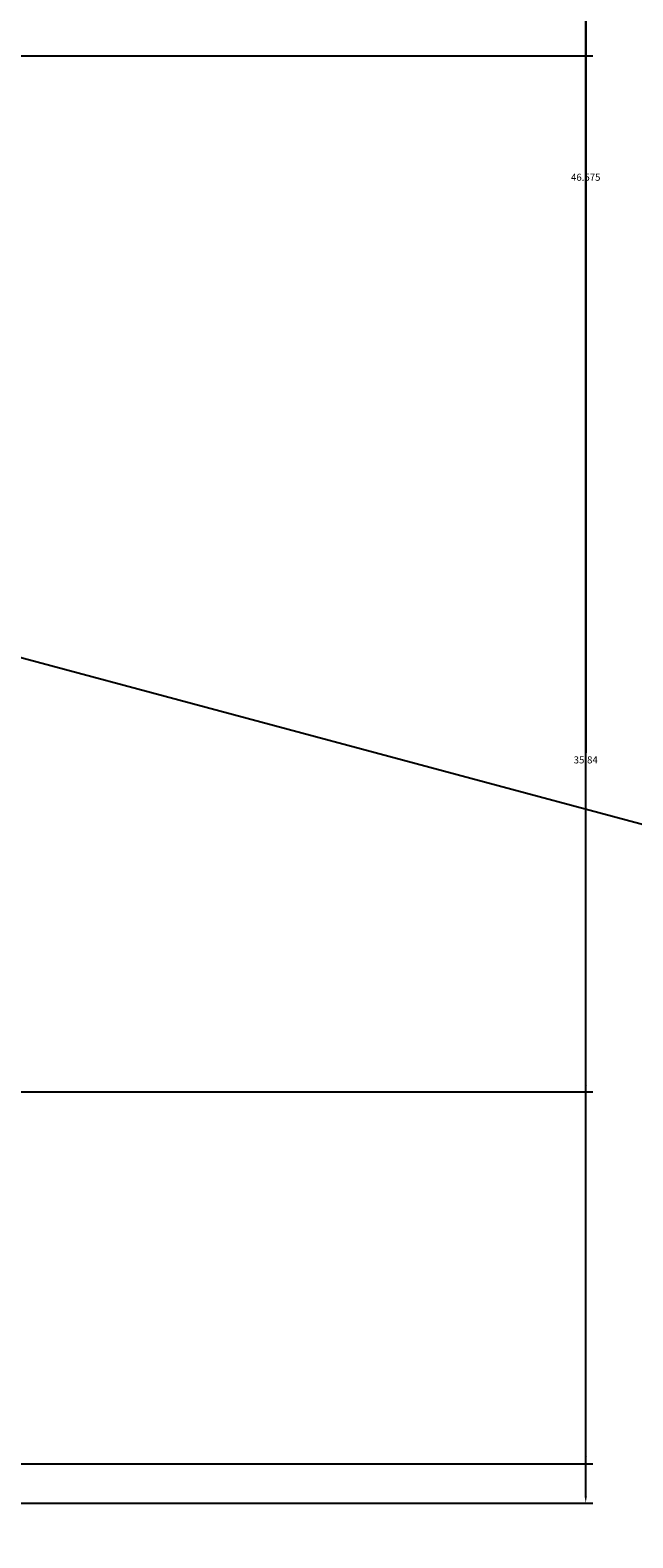
# Model space of a CAD drawing. Units: inches. Extents: x -12 to 334, y -10 to 186.
# Tile 72 of 77: x 282 to 297, y 45 to 83. Entities that reach past the tile are written whole.
import ezdxf
from ezdxf import colors
from ezdxf.entities.mleader import LeaderData, LeaderLine
from ezdxf.math import Vec2, Vec3

# ---------------------------------------------------------------- set-up
doc = ezdxf.new("R2010")
doc.units = ezdxf.units.IN
doc.header["$MEASUREMENT"] = 0
doc.layers.add('M-ANNO-TEXT', color=3, linetype='Continuous', lineweight=25)
doc.layers.add('M-DIMS', color=2, linetype='Continuous', lineweight=18)
doc.styles.get("Standard").update_dxf_attribs({"font": 'arial.ttf'})
doc.dimstyles.get("Standard").update_dxf_attribs({"dimtxt": 0.18, "dimasz": 0.18, "dimexe": 0.18, "dimexo": 0.0625, "dimgap": 0.09, "dimtad": 0, "dimtih": 1, "dimtoh": 1, "dimdec": 4, "dimzin": 0, "dimdsep": 46, "dimtxsty": 'Standard', "dimcen": 0.09, "dimadec": 0, "dimazin": 0, "dimtfac": 1, "dimtdec": 4, "dimtofl": 0, "dimtmove": 0, "dimatfit": 3, "dimfxl": 1, "dimtolj": 1, "dimtzin": 0, "dimarcsym": 0})

# ---------------------------------------------------------------- blocks, each defined once
blk = doc.blocks.new('*D17')
at = {"layer": 'Defpoints', "color": 0, "transparency": 16777216}
for p in [(106.177, 102.896), (105.892, 56.321), (295.976, 56.321)]:
    blk.add_point(p, dxfattribs=at)
at = {"layer": 'M-DIMS', "color": 0, "lineweight": -2, "transparency": 16777216}
for p, q in [((106.24, 102.896), (296.156, 102.896)), ((295.976, 102.716), (295.976, 79.79)), ((295.976, 56.501), (295.976, 79.426)), ((105.954, 56.321), (296.156, 56.321))]:
    blk.add_line(p, q, dxfattribs=at)
at = {"layer": 'M-DIMS', "color": 0, "transparency": 16777216}
for points in [[(295.946, 102.716), (296.006, 102.716), (295.976, 102.896)], [(295.946, 56.501), (296.006, 56.501), (295.976, 56.321)]]:
    blk.add_solid(points, dxfattribs=at)
at = {"layer": 'M-DIMS', "color": 0, "transparency": 16777216, "insert": (295.976, 79.608), "char_height": 0.18, "attachment_point": 5}
blk.add_mtext('\\A1;46.575', dxfattribs=at)
blk = doc.blocks.new('*D24')
at = {"layer": 'Defpoints', "color": 0, "transparency": 16777216}
for p in [(269.381, 137.943), (269.381, 45.854), (295.976, 45.854)]:
    blk.add_point(p, dxfattribs=at)
at = {"layer": 'M-DIMS', "color": 0, "lineweight": -2, "transparency": 16777216}
for p, q in [((269.443, 137.943), (296.156, 137.943)), ((295.976, 137.763), (295.976, 92.081)), ((295.976, 46.034), (295.976, 91.717)), ((269.443, 45.854), (296.156, 45.854))]:
    blk.add_line(p, q, dxfattribs=at)
at = {"layer": 'M-DIMS', "color": 0, "transparency": 16777216}
for points in [[(295.946, 137.763), (296.006, 137.763), (295.976, 137.943)], [(295.946, 46.034), (296.006, 46.034), (295.976, 45.854)]]:
    blk.add_solid(points, dxfattribs=at)
at = {"layer": 'M-DIMS', "color": 0, "transparency": 16777216, "insert": (295.976, 91.899), "char_height": 0.18, "attachment_point": 5}
blk.add_mtext('\\A1;92.09', dxfattribs=at)
blk = doc.blocks.new('*D38')
at = {"layer": 'Defpoints', "color": 0, "transparency": 16777216}
for p in [(247.935, 82.697), (247.935, 46.854), (295.976, 46.854)]:
    blk.add_point(p, dxfattribs=at)
at = {"layer": 'M-DIMS', "color": 0, "lineweight": -2, "transparency": 16777216}
for p, q in [((247.998, 82.697), (296.156, 82.697)), ((295.976, 82.517), (295.976, 64.957)), ((295.976, 47.034), (295.976, 64.594)), ((247.998, 46.854), (296.156, 46.854))]:
    blk.add_line(p, q, dxfattribs=at)
at = {"layer": 'M-DIMS', "color": 0, "transparency": 16777216}
for points in [[(295.946, 82.517), (296.006, 82.517), (295.976, 82.697)], [(295.946, 47.034), (296.006, 47.034), (295.976, 46.854)]]:
    blk.add_solid(points, dxfattribs=at)
at = {"layer": 'M-DIMS', "color": 0, "transparency": 16777216, "insert": (295.976, 64.775), "char_height": 0.18, "attachment_point": 5}
blk.add_mtext('\\A1;35.84', dxfattribs=at)
blk = doc.blocks.new('*D41')
at = {"layer": 'Defpoints', "color": 0, "transparency": 16777216}
for p in [(190.169, 91.899), (277.343, 68.515)]:
    blk.add_point(p, dxfattribs=at)
at = {"layer": 'M-DIMS', "color": 0, "lineweight": -2, "transparency": 16777216}
for p, q in [((190.079, 91.899), (190.259, 91.899)), ((190.169, 91.809), (190.169, 91.989)), ((329.648, 54.485), (277.517, 68.469)), ((329.828, 54.485), (329.648, 54.485))]:
    blk.add_line(p, q, dxfattribs=at)
at = {"layer": 'M-DIMS', "color": 0, "transparency": 16777216}
blk.add_solid([(277.525, 68.498), (277.509, 68.44), (277.343, 68.515)], dxfattribs=at)
at = {"layer": 'M-DIMS', "color": 0, "transparency": 16777216, "insert": (330.307, 54.485), "char_height": 0.18, "attachment_point": 5}
blk.add_mtext('\\A1;R90.26', dxfattribs=at)

msp = doc.modelspace()

# ---------------------------------------------------------------- dimensions: what is measured, and where the dimension line sits
at = {"layer": 'M-DIMS'}
for base, p1, p2, override, picture, middle in [((295.9756, 45.8541), (269.3808, 137.9435), (269.3808, 45.8541), {"dimdec": 2, "dimlfac": 1, "dimrnd": 0, "dimzin": 0, "dimdsep": 46, "dimlunit": 2}, '*D24', (295.9756, 91.8988)), ((295.9756, 56.3205), (106.1771, 102.8958), (105.8919, 56.3205), {"dimdec": 3, "dimlfac": 1, "dimrnd": 0, "dimzin": 0, "dimdsep": 46, "dimlunit": 2}, '*D17', (295.9756, 79.6082)), ((295.9756, 46.8541), (247.9354, 82.6969), (247.9354, 46.8541), {"dimdec": 2, "dimlfac": 1, "dimrnd": 0, "dimzin": 0, "dimdsep": 46, "dimlunit": 2}, '*D38', (295.9756, 64.7755))]:
    dim = msp.add_linear_dim(base=base, p1=p1, p2=p2, angle=90, dimstyle='Standard', override=override, dxfattribs=at)
    dim.commit()
    dim.dimension.update_dxf_attribs({"geometry": picture, "text_midpoint": middle})
dim = msp.add_radius_dim(center=(190.1689, 91.8988), mpoint=(277.3431, 68.5153), dimstyle='Standard', override={"dimdec": 2, "dimlfac": 1, "dimrnd": 0, "dimzin": 0, "dimdsep": 46, "dimlunit": 2}, dxfattribs=at)
dim.commit()
dim.dimension.update_dxf_attribs({"geometry": '*D41', "text_midpoint": (330.3074, 54.4851), "dimtype": 164})

# ---------------------------------------------------------------- leaders
at = {"layer": 'M-ANNO-TEXT'}
ml = msp.add_multileader_mtext('Standard', dxfattribs=at)
ml.set_content('^I^IWeir', color=256)
ml.set_leader_properties()
ml.build(insert=Vec2(0, 0))
ml.multileader.update_dxf_attribs({"dogleg_length": 0.36, "arrow_head_size": 0.7})
ctx = ml.context
ctx.base_point, ctx.arrow_head_size, ctx.landing_gap_size, ctx.plane_origin = Vec3(257.1525, 34.1955), 0.7, 0.09, Vec3(247.9354, 49.9015)
notes = []
notes.append((ctx, [(0, (1, 1, 0), (255.3593, 34.1955), (1, 0), 1.7932, [(0, [(247.9354, 49.9015)], 0, [])])]))
ctx.mtext.insert, ctx.mtext.flow_direction = Vec3(257.2425, 36.2283), 5
for ctx, leaders in notes:
    for number, flags, end, landing, length, lines in leaders:
        leader = LeaderData()
        leader.index, (leader.has_last_leader_line, leader.has_dogleg_vector, leader.attachment_direction) = number, flags
        leader.last_leader_point, leader.dogleg_vector, leader.dogleg_length = Vec3(end), Vec3(landing), length
        for number, points, colour, breaks in lines:
            line = LeaderLine()
            line.index, line.vertices, line.color, line.breaks = number, Vec3.list(points), colors.encode_raw_color(colour), breaks
            leader.lines.append(line)
        ctx.leaders.append(leader)

doc.saveas('drawing.dxf')
